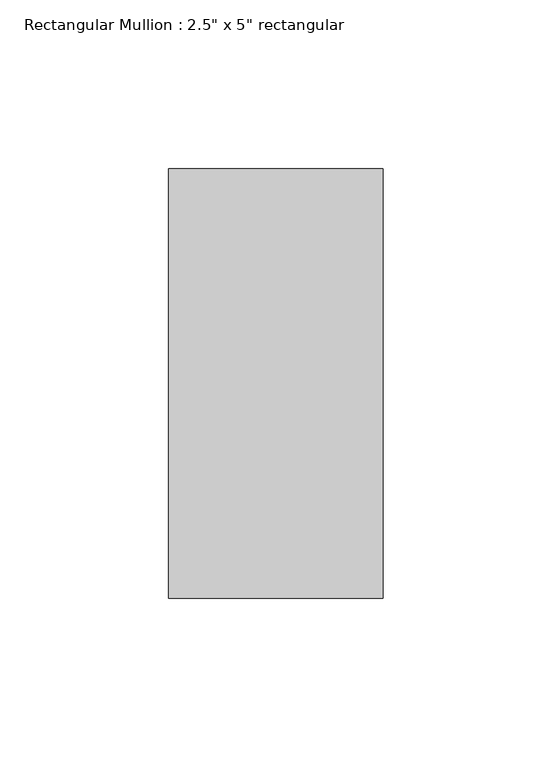
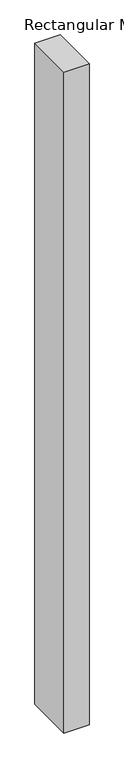
"""IFC4 building model written with IfcOpenShell, lengths in millimetres: member geometry."""

from ifc_helpers import new_model, si_unit, frame, origin, place, context, project, spatial, polyline, outline, extrude, source, transform, mapped, element, save


def member_6d5c3e5e(model_context):
    return source(origin(), model_context, "Body", "SweptSolid", [
        extrude(outline(polyline([(0.0, 63.5), (0.0, -63.5), (-63.5, -63.5), (-63.5, 63.5), (0.0, 63.5)])), frame((0.0, 0.0, -1765.3), z_axis=(0.0, 0.0, 1.0), x_axis=(1.0, 0.0, 0.0)), (0.0, 0.0, 1.0), 1765.3),
    ])


if __name__ == "__main__":
    model = new_model("IFC4")
    model_context = context("Model", 3, world=origin())
    ifc_project = project(units=[si_unit("LENGTHUNIT", "METRE", prefix="MILLI")], contexts=[model_context])
    site = spatial("IfcSite", under=ifc_project)
    building = spatial("IfcBuilding", under=site)
    placement = place(None, origin())
    member_shape = member_6d5c3e5e(model_context)
    element("IfcMember", 1, ObjectType="Rectangular Mullion : 2.5\" x 5\" rectangular", at=placement, inside=building, context=model_context, shape_type="MappedRepresentation", body=[
        mapped(member_shape, transform((0.0, 0.0, 0.0), x_axis=(1.0, 0.0, 0.0), y_axis=(0.0, 1.0, 0.0), z_axis=(0.0, 0.0, 1.0))),
    ])
    save(model, "model.ifc")

# Revit data of these elements
# Type "Rectangular Mullion : 2.5\" x 5\" rectangular"
#   built-in parameter 1007304 = 0.416667 (stored number, unit not read)
#   built-in parameter 1007301 = 0.104167 (stored number, unit not read)
#   built-in parameter 1007300 = 0.104167 (stored number, unit not read)
# Element 1 (IfcMember, "Rectangular Mullion : 2.5\" x 5\" rectangular")
#   Materials on its faces: "Aluminum"
# Materials
#   "Aluminum": class "Metal", colour RGB 247 247 247, transparency 0, Description = "Aluminum 6061", Cost = 0
